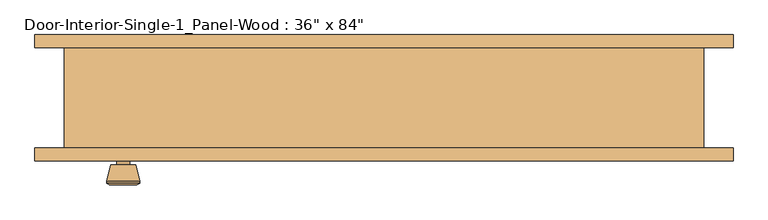
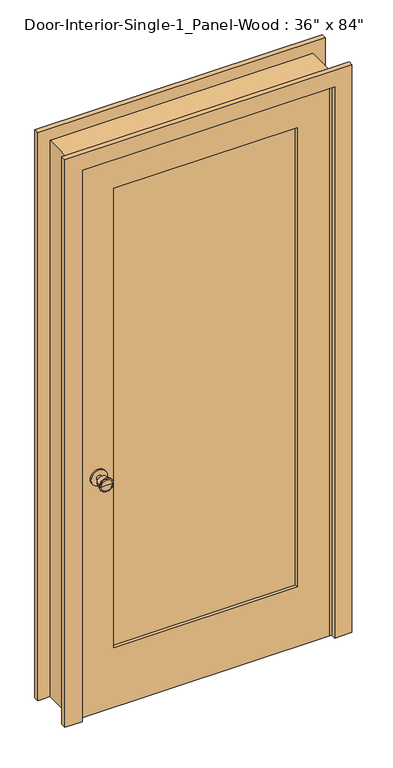
"""IFC4 building model written with IfcOpenShell, lengths in millimetres: door geometry."""

from ifc_helpers import new_model, si_unit, point, frame, frame_2d, origin, place, context, project, spatial, polyline, circle_curve, trimmed, segment, composite_curve, outline, extrude, faceted_brep, source, transform, mapped, element, save
from ifc_brep_helpers import plane_surface, cylinder_surface, revolved_surface, advanced_brep


def door_5a860750(model_context):
    return source(origin(), model_context, "Body", "SolidModel", [
        advanced_brep(
        [(-393.7, -32.1, 914.4), (-403.7, -32.1, 914.4), (-383.7, -32.1, 914.4), (-373.2241324, 16.9, 914.4), (-414.1758676, 16.9, 914.4), (-393.7, 16.9, 914.4), (-368.7, 15.0721319, 914.4), (-418.7, 15.0721319, 914.4), (-368.7, 11.6084537, 914.4), (-418.7, 11.6084537, 914.4), (-375.063764, -13.1, 914.4), (-412.336236, -13.1, 914.4), (-383.7, -13.1, 914.4), (-403.7, -13.1, 914.4)],
        [
            (0, 1),
            (1, 2, circle_curve(frame((-393.7, -32.1, 914.4), z_axis=(0.0, -1.0, 0.0), x_axis=(-1.0, 0.0, 0.0)), 10.0)),
            (2, 0),
            (2, 1, circle_curve(frame((-393.7, -32.1, 914.4), z_axis=(0.0, -1.0, 0.0), x_axis=(-1.0, 0.0, 0.0)), 10.0)),
            (3, 4, circle_curve(frame((-393.7, 16.9, 914.4), z_axis=(0.0, 1.0, 0.0), x_axis=(-1.0, 0.0, 0.0)), 20.4758676)),
            (4, 5),
            (5, 3),
            (4, 3, circle_curve(frame((-393.7, 16.9, 914.4), z_axis=(0.0, 1.0, 0.0), x_axis=(-1.0, 0.0, 0.0)), 20.4758676)),
            (6, 7, circle_curve(frame((-393.7, 15.0721319, 914.4), z_axis=(0.0, 1.0, 0.0), x_axis=(-1.0, 0.0, 0.0)), 25.0)),
            (7, 4),
            (3, 6),
            (7, 6, circle_curve(frame((-393.7, 15.0721319, 914.4), z_axis=(0.0, 1.0, 0.0), x_axis=(-1.0, 0.0, 0.0)), 25.0)),
            (8, 9, circle_curve(frame((-393.7, 11.6084537, 914.4), z_axis=(0.0, 1.0, 0.0), x_axis=(-1.0, 0.0, 0.0)), 25.0)),
            (9, 7),
            (6, 8),
            (9, 8, circle_curve(frame((-393.7, 11.6084537, 914.4), z_axis=(0.0, 1.0, 0.0), x_axis=(-1.0, 0.0, 0.0)), 25.0)),
            (10, 11, circle_curve(frame((-393.7, -13.1, 914.4), z_axis=(0.0, 1.0, 0.0), x_axis=(-1.0, 0.0, 0.0)), 18.636236)),
            (11, 9),
            (8, 10),
            (11, 10, circle_curve(frame((-393.7, -13.1, 914.4), z_axis=(0.0, 1.0, 0.0), x_axis=(-1.0, 0.0, 0.0)), 18.636236)),
            (12, 13, circle_curve(frame((-393.7, -13.1, 914.4), z_axis=(0.0, 1.0, 0.0), x_axis=(-1.0, 0.0, 0.0)), 10.0)),
            (13, 11),
            (10, 12),
            (13, 12, circle_curve(frame((-393.7, -13.1, 914.4), z_axis=(0.0, 1.0, 0.0), x_axis=(-1.0, 0.0, 0.0)), 10.0)),
            (1, 13),
            (12, 2),
        ],
        [
            plane_surface(frame((-393.7, -32.1, 914.4), z_axis=(0.0, -1.0, 0.0), x_axis=(-1.0, 0.0, 0.0))),
            plane_surface(frame((-393.7, 16.9, 914.4), z_axis=(0.0, 1.0, 0.0), x_axis=(-1.0, 0.0, 0.0))),
            revolved_surface(polyline([(-414.1758676, 16.9, 914.4), (-418.7, 15.0721319, 914.4)]), (-393.7, -32.1, 914.4), (0.0, -1.0, 0.0)),
            cylinder_surface(frame((-393.7, -32.1, 914.4), z_axis=(0.0, -1.0, 0.0), x_axis=(-1.0, 0.0, 0.0)), 25.0),
            revolved_surface(polyline([(-418.7, 11.6084537, 914.4), (-412.336236, -13.1, 914.4)]), (-393.7, -32.1, 914.4), (0.0, -1.0, 0.0)),
            plane_surface(frame((-393.7, -13.1, 914.4), z_axis=(0.0, -1.0, 0.0), x_axis=(-1.0, 0.0, 0.0))),
            cylinder_surface(frame((-393.7, -32.1, 914.4), z_axis=(0.0, -1.0, 0.0), x_axis=(-1.0, 0.0, 0.0)), 10.0),
        ],
        [
            (0, [[1, 2, 3]]),
            (0, [[-3, 4, -1]]),
            (1, [[5, 6, 7]]),
            (1, [[8, -7, -6]]),
            (2, [[9, 10, -5, 11]]),
            (2, [[12, -11, -8, -10]]),
            (3, [[13, 14, -9, 15]]),
            (3, [[16, -15, -12, -14]]),
            (4, [[17, 18, -13, 19]]),
            (4, [[20, -19, -16, -18]]),
            (5, [[21, 22, -17, 23]]),
            (5, [[24, -23, -20, -22]]),
            (6, [[-2, 25, -21, 26]]),
            (6, [[-4, -26, -24, -25]]),
        ],
    ),
        extrude(outline(composite_curve([segment(trimmed(circle_curve(frame_2d((914.4, -393.7)), 30.0), [point((914.4, -423.7))], [point((914.4, -363.7))], False, "CARTESIAN"), True, "CONTINUOUS"), segment(trimmed(circle_curve(frame_2d((914.4, -393.7)), 30.0), [point((914.4, -363.7))], [point((914.4, -423.7))], False, "CARTESIAN"), True, "CONTINUOUS")], self_intersect=False)), frame((0.0, -38.1, 0.0), z_axis=(0.0, 1.0, 0.0), x_axis=(0.0, 0.0, 1.0)), (0.0, 0.0, 1.0), 6.0),
        advanced_brep(
        [(-393.7, -79.025, 914.4), (-383.7, -79.025, 914.4), (-403.7, -79.025, 914.4), (-373.2241324, -128.025, 914.4), (-393.7, -128.025, 914.4), (-414.1758676, -128.025, 914.4), (-368.7, -126.1971319, 914.4), (-418.7, -126.1971319, 914.4), (-368.7, -122.7334537, 914.4), (-418.7, -122.7334537, 914.4), (-375.063764, -98.025, 914.4), (-412.336236, -98.025, 914.4), (-383.7, -98.025, 914.4), (-403.7, -98.025, 914.4)],
        [
            (0, 1),
            (1, 2, circle_curve(frame((-393.7, -79.025, 914.4), z_axis=(0.0, 1.0, 0.0), x_axis=(-1.0, 0.0, 0.0)), 10.0)),
            (2, 0),
            (2, 1, circle_curve(frame((-393.7, -79.025, 914.4), z_axis=(0.0, 1.0, 0.0), x_axis=(-1.0, 0.0, 0.0)), 10.0)),
            (3, 4),
            (4, 5),
            (5, 3, circle_curve(frame((-393.7, -128.025, 914.4), z_axis=(0.0, -1.0, 0.0), x_axis=(-1.0, 0.0, 0.0)), 20.4758676)),
            (3, 5, circle_curve(frame((-393.7, -128.025, 914.4), z_axis=(0.0, -1.0, 0.0), x_axis=(-1.0, 0.0, 0.0)), 20.4758676)),
            (6, 3),
            (5, 7),
            (7, 6, circle_curve(frame((-393.7, -126.1971319, 914.4), z_axis=(0.0, -1.0, 0.0), x_axis=(-1.0, 0.0, 0.0)), 25.0)),
            (6, 7, circle_curve(frame((-393.7, -126.1971319, 914.4), z_axis=(0.0, -1.0, 0.0), x_axis=(-1.0, 0.0, 0.0)), 25.0)),
            (8, 6),
            (7, 9),
            (9, 8, circle_curve(frame((-393.7, -122.7334537, 914.4), z_axis=(0.0, -1.0, 0.0), x_axis=(-1.0, 0.0, 0.0)), 25.0)),
            (8, 9, circle_curve(frame((-393.7, -122.7334537, 914.4), z_axis=(0.0, -1.0, 0.0), x_axis=(-1.0, 0.0, 0.0)), 25.0)),
            (10, 8),
            (9, 11),
            (11, 10, circle_curve(frame((-393.7, -98.025, 914.4), z_axis=(0.0, -1.0, 0.0), x_axis=(-1.0, 0.0, 0.0)), 18.636236)),
            (10, 11, circle_curve(frame((-393.7, -98.025, 914.4), z_axis=(0.0, -1.0, 0.0), x_axis=(-1.0, 0.0, 0.0)), 18.636236)),
            (12, 10),
            (11, 13),
            (13, 12, circle_curve(frame((-393.7, -98.025, 914.4), z_axis=(0.0, -1.0, 0.0), x_axis=(-1.0, 0.0, 0.0)), 10.0)),
            (12, 13, circle_curve(frame((-393.7, -98.025, 914.4), z_axis=(0.0, -1.0, 0.0), x_axis=(-1.0, 0.0, 0.0)), 10.0)),
            (1, 12),
            (13, 2),
        ],
        [
            plane_surface(frame((-393.7, -79.025, 914.4), z_axis=(0.0, 1.0, 0.0), x_axis=(-1.0, 0.0, 0.0))),
            plane_surface(frame((-393.7, -128.025, 914.4), z_axis=(0.0, -1.0, 0.0), x_axis=(-1.0, 0.0, 0.0))),
            revolved_surface(polyline([(-414.1758676, -128.025, 914.4), (-418.7, -126.1971319, 914.4)]), (-393.7, -79.025, 914.4), (0.0, 1.0, 0.0)),
            cylinder_surface(frame((-393.7, -79.025, 914.4), z_axis=(0.0, 1.0, 0.0), x_axis=(-1.0, 0.0, 0.0)), 25.0),
            revolved_surface(polyline([(-418.7, -122.7334537, 914.4), (-412.336236, -98.025, 914.4)]), (-393.7, -79.025, 914.4), (0.0, 1.0, 0.0)),
            plane_surface(frame((-393.7, -98.025, 914.4), z_axis=(0.0, 1.0, 0.0), x_axis=(-1.0, 0.0, 0.0))),
            cylinder_surface(frame((-393.7, -79.025, 914.4), z_axis=(0.0, 1.0, 0.0), x_axis=(-1.0, 0.0, 0.0)), 10.0),
        ],
        [
            (0, [[1, 2, 3]]),
            (0, [[-3, 4, -1]]),
            (1, [[5, 6, 7]]),
            (1, [[-6, -5, 8]]),
            (2, [[9, -7, 10, 11]]),
            (2, [[-10, -8, -9, 12]]),
            (3, [[13, -11, 14, 15]]),
            (3, [[-14, -12, -13, 16]]),
            (4, [[17, -15, 18, 19]]),
            (4, [[-18, -16, -17, 20]]),
            (5, [[21, -19, 22, 23]]),
            (5, [[-22, -20, -21, 24]]),
            (6, [[25, -23, 26, -2]]),
            (6, [[-26, -24, -25, -4]]),
        ],
    ),
        extrude(outline(composite_curve([segment(trimmed(circle_curve(frame_2d((914.4, -393.7)), 30.0), [point((914.4, -423.7))], [point((914.4, -363.7))], False, "CARTESIAN"), True, "CONTINUOUS"), segment(trimmed(circle_curve(frame_2d((914.4, -393.7)), 30.0), [point((914.4, -363.7))], [point((914.4, -423.7))], False, "CARTESIAN"), True, "CONTINUOUS")], self_intersect=False)), frame((0.0, -79.025, 0.0), z_axis=(0.0, 1.0, 0.0), x_axis=(0.0, 0.0, 1.0)), (0.0, 0.0, 1.0), 6.0),
        faceted_brep([(482.6, -73.025, 0.0), (457.2, -73.025, 0.0), (457.2, -38.1, 0.0), (444.5, -38.1, 0.0), (444.5, -3.175, 0.0), (457.2, -3.175, 0.0), (457.2, 79.375, 0.0), (482.6, 79.375, 0.0), (482.6, 79.375, 2159.0), (482.6, -73.025, 2159.0), (457.2, 79.375, 2133.6), (-457.2, 79.375, 2133.6), (-457.2, 79.375, 0.0), (-482.6, 79.375, 0.0), (-482.6, 79.375, 2159.0), (457.2, -3.175, 2133.6), (444.5, -3.175, 2120.9), (-444.5, -3.175, 2120.9), (-444.5, -3.175, 0.0), (-457.2, -3.175, 0.0), (-457.2, -3.175, 2133.6), (444.5, -38.1, 2120.9), (457.2, -38.1, 2133.6), (-457.2, -38.1, 2133.6), (-457.2, -38.1, 0.0), (-444.5, -38.1, 0.0), (-444.5, -38.1, 2120.9), (457.2, -73.025, 2133.6), (-482.6, -73.025, 2159.0), (-482.6, -73.025, 0.0), (-457.2, -73.025, 0.0), (-457.2, -73.025, 2133.6)], [[[0, 1, 2, 3, 4, 5, 6, 7]], [[7, 8, 9, 0]], [[6, 10, 11, 12, 13, 14, 8, 7]], [[5, 15, 10, 6]], [[4, 16, 17, 18, 19, 20, 15, 5]], [[3, 21, 16, 4]], [[2, 22, 23, 24, 25, 26, 21, 3]], [[1, 27, 22, 2]], [[0, 9, 28, 29, 30, 31, 27, 1]], [[8, 14, 28, 9]], [[15, 20, 11, 10]], [[21, 26, 17, 16]], [[27, 31, 23, 22]], [[29, 13, 12, 19, 18, 25, 24, 30]], [[14, 13, 29, 28]], [[20, 19, 12, 11]], [[26, 25, 18, 17]], [[31, 30, 24, 23]]]),
        extrude(outline(polyline([(2133.6, -457.2), (0.0, -457.2), (0.0, 457.2), (2133.6, 457.2), (2133.6, -457.2)]), holes=[polyline([(2014.5375, -336.55), (2014.5375, 336.55), (231.775, 336.55), (231.775, -336.55), (2014.5375, -336.55)])]), frame((0.0, -73.025, 0.0), z_axis=(0.0, 1.0, 0.0), x_axis=(0.0, 0.0, 1.0)), (0.0, 0.0, 1.0), 34.925),
        extrude(outline(polyline([(336.55, -49.7416667), (336.55, -61.3833333), (-336.55, -61.3833333), (-336.55, -49.7416667), (336.55, -49.7416667)])), frame((0.0, 0.0, 231.775), z_axis=(0.0, 0.0, 1.0), x_axis=(1.0, 0.0, 0.0)), (0.0, 0.0, 1.0), 1782.7625),
        extrude(outline(polyline([(0.0, 527.05), (2203.45, 527.05), (2203.45, -527.05), (0.0, -527.05), (0.0, -463.55), (2139.95, -463.55), (2139.95, 463.55), (0.0, 463.55), (0.0, 527.05)])), frame((0.0, -92.075, 0.0), z_axis=(0.0, 1.0, 0.0), x_axis=(0.0, 0.0, 1.0)), (0.0, 0.0, 1.0), 19.05),
        extrude(outline(polyline([(0.0, 527.05), (2203.45, 527.05), (2203.45, -527.05), (0.0, -527.05), (0.0, -463.55), (2139.95, -463.55), (2139.95, 463.55), (0.0, 463.55), (0.0, 527.05)])), frame((0.0, 79.375, 0.0), z_axis=(0.0, 1.0, 0.0), x_axis=(0.0, 0.0, 1.0)), (0.0, 0.0, 1.0), 19.05),
    ])


if __name__ == "__main__":
    model = new_model("IFC4")
    model_context = context("Model", 3, world=origin())
    ifc_project = project(units=[si_unit("LENGTHUNIT", "METRE", prefix="MILLI")], contexts=[model_context])
    site = spatial("IfcSite", under=ifc_project)
    building = spatial("IfcBuilding", under=site)
    placement = place(None, origin())
    door_shape = door_5a860750(model_context)
    element("IfcDoor", 1, ObjectType="Door-Interior-Single-1_Panel-Wood : 36\" x 84\"", at=placement, inside=building, context=model_context, shape_type="MappedRepresentation", body=[
        mapped(door_shape, transform((0.0, 0.0, 0.0), x_axis=(1.0, 0.0, 0.0), y_axis=(0.0, 1.0, 0.0), z_axis=(0.0, 0.0, 1.0))),
    ])
    save(model, "model.ifc")

# Revit data of these elements
# Type "Door-Interior-Single-1_Panel-Wood : 36\" x 84\""
#   Type Mark = "8"
#   Assembly Code = "C1020300"
#   Analytic Construction = "Wooden"
#   Top Rail = 0' - 4 11/16"
#   Thickness = 0' - 1 3/8"
#   Thermal Resistance (R) = 2.5876 (h·ft²·°F)/BTU
#   Swing Angle [instance default] = 90.00°
#   Stiles = 0' - 4 3/4"
#   Rough Width = 3' - 2"
#   Rough Height = 7' - 1"
#   Height = 7' - 0"
#   Width = 3' - 0"
#   Heat Transfer Coefficient (U) = 0.3865 BTU/(h·ft²·°F)
#   Bottom Rail = 0' - 9 1/8"
#   Trim Material = Cherry
#   Panel Material = Cherry
#   Frame Material = Cherry
#   Door Handle Material = Aluminum
#   Visual Light Transmittance = 0
#   Solar Heat Gain Coefficient = 0
#   Wall Closure = (empty or 0)
#   Function = (empty or 0)
# Element 1 (IfcDoor, "Door-Interior-Single-1_Panel-Wood : 36\" x 84\"")
#   Materials on its faces: "Cherry", "Aluminum"
# Materials
#   "Cherry": class "Wood", colour RGB 226 177 128, transparency 0, Description = "Prunus Serotina", Cost = 0
#   "Aluminum": class "Metal", colour RGB 247 247 247, transparency 0, Description = "Aluminum 6061", Cost = 0
